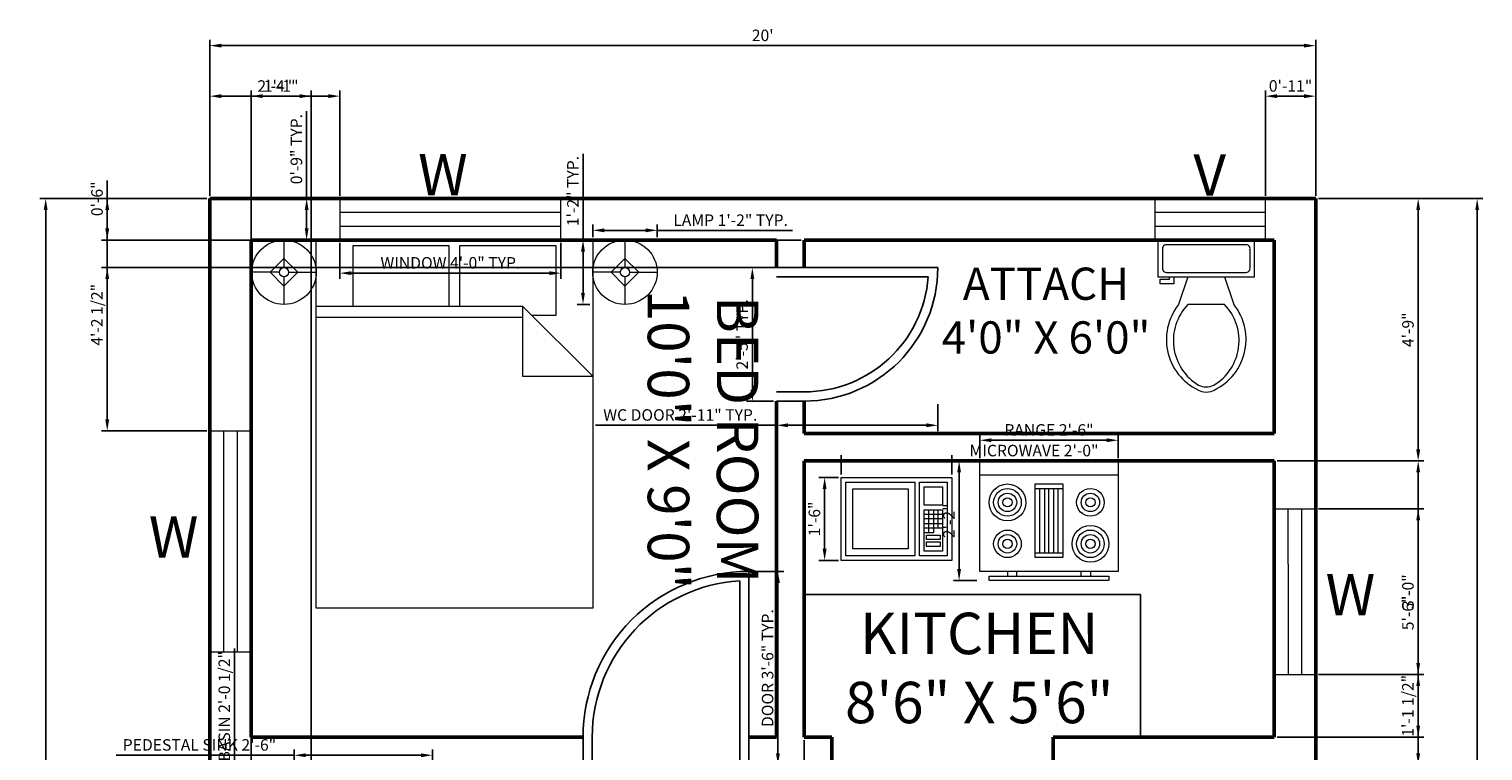
# Model space of a CAD drawing. Units: inches. Extents: x 2530 to 2846, y 1711 to 2145.
# Tile 3 of 3: x 2530 to 2846, y 1989 to 2145. Entities that reach past the tile are written whole.
import ezdxf

# ---------------------------------------------------------------- set-up
doc = ezdxf.new("R2010")
doc.units = ezdxf.units.IN
for name, color, linetype, lineweight in [('A-ANNO-DIMS', 2, 'Continuous', 18), ('A-ANNO-TEXT', 7, 'Continuous', 18), ('A-AREA-IDEN', 7, 'Continuous', 25), ('A-DOOR', 3, 'Continuous', 25), ('A-EQPM', 8, 'Continuous', 18), ('A-FLOR-CASE', 8, 'Continuous', 25), ('A-FLOR-FIXT', 9, 'Continuous', 18), ('A-FURN', 8, 'Continuous', 18), ('A-GLAZ', 4, 'Continuous', 18), ('A-WALL', 7, 'Continuous', 50)]:
    doc.layers.add(name, color=color, linetype=linetype, lineweight=lineweight)
doc.styles.get("Standard").update_dxf_attribs({"font": 'arial.ttf'})
doc.dimstyles.new('ISO-25', dxfattribs={"dimtxt": 2.5, "dimasz": 2.5, "dimexe": 1.25, "dimexo": 0.625, "dimtad": 1, "dimdec": 0, "dimlunit": 3, "dimtxsty": 'Standard', "dimcen": 2.5, "dimadec": 0, "dimazin": 0, "dimtfac": 1, "dimtdec": 0, "dimtmove": 0, "dimatfit": 3, "dimfxl": 1, "dimarcsym": 0})

# ---------------------------------------------------------------- blocks, each defined once
blk = doc.blocks.new('Toilet - top')
for p, q in [((9.5, -6), (9.5, -2)), ((-10, -8.5), (-8, -8.5)), ((-10, -9.5), (-10, -8.5)), ((-8, -8.5), (-8, -8)), ((-7, -8), (-7, -9.5)), ((-4, -8), (-6, -14)), ((4, -8), (6, -14)), ((-7, -9.5), (-10, -9.5)), ((4, -14), (-4, -14))]:
    blk.add_line(p, q)
blk.add_lwpolyline([(10.5, -8), (10.5, 0), (-10.5, 0), (-10.5, -8)], close=True)
for points in [[(-9.5, -2), (-9.5, -6)], [(8.5, -1), (-8.5, -1)], [(-8.5, -7), (8.5, -7)]]:
    blk.add_lwpolyline(points)
for centre, radius, start, end in [((-8.62, -1.88), 0.884, 81.8699, 188.1301), ((8.62, -1.88), 0.884, 351.8699, 98.1301), ((-8.62, -6.12), 0.884, 171.8699, 278.1301), ((8.62, -6.12), 0.884, 261.8699, 8.1301), ((3.52, -21.58), 12.17, 141.4691, 247.9714), ((4.2, -21.82), 11.33, 136.3677, 238.9468), ((-3.52, -21.58), 12.17, 292.0284, 38.5307), ((-4.2, -21.82), 11.33, 301.053, 43.6321), ((0, -27.88), 4, 245.7318, 294.2682), ((0, -29), 4, 254.8605, 285.1395)]:
    blk.add_arc(centre, radius, start, end)
blk = doc.blocks.new('Bed - Queen')
for p, q in [((0, -80.00003), (0, 0)), ((0, 0), (59.99999, 0)), ((59.99999, 0), (59.99999, -80.00003)), ((7.99999, -1.2), (28.79998, -1.2)), ((7.99999, -14.4), (7.99999, -1.2)), ((28.79998, -1.2), (28.79998, -14.4)), ((31.19999, -1.2), (51.99999, -1.2)), ((31.19999, -14.4), (31.19999, -1.2)), ((51.99999, -1.2), (51.99999, -16.4)), ((0, -14.4), (44.8, -14.4)), ((59.99999, -29.6), (44.8, -14.4)), ((44.8, -14.4), (44.8, -29.6)), ((44.8, -16.8), (0, -16.8)), ((51.99999, -16.4), (46.79936, -16.4)), ((44.8, -29.6), (59.99999, -29.6)), ((59.99999, -80.00003), (0, -80.00003))]:
    blk.add_line(p, q)
blk = doc.blocks.new('Lamp - Table')
for p, q in [((0, 7), (0, 1)), ((-1, 0), (-7, 0)), ((0, 3), (-3, 0)), ((-3, 0), (0, -3)), ((3, 0), (0, 3)), ((0, -3), (3, 0)), ((1, 0), (7, 0)), ((0, -1), (0, -7))]:
    blk.add_line(p, q)
for radius in [7, 1]:
    blk.add_circle((0, 0), radius)
blk = doc.blocks.new('Range-Oven - 30 in top')
for p, q in [((0, -3), (30, -3)), ((12, -6), (18, -6)), ((13, -20), (13, -6)), ((14, -6), (14, -20)), ((15, -20), (15, -6)), ((16, -6), (16, -20)), ((17, -20), (17, -6)), ((18, -20), (12, -20)), ((6, -24), (6, -25)), ((8, -25), (8, -24)), ((22, -25), (22, -24)), ((24, -24), (24, -25))]:
    blk.add_line(p, q)
for points in [[(0, -24), (0, 0), (30, 0), (30, -24)], [(12, -21), (12, -5), (18, -5), (18, -21)], [(2, -26), (2, -25), (28, -25), (28, -26)]]:
    blk.add_lwpolyline(points, close=True)
for centre, radius in [((6, -9), 4), ((6, -9), 3), ((24, -9), 3), ((6, -9), 2), ((6, -9), 1), ((24, -9), 2), ((24, -9), 1), ((6, -18), 3), ((24, -18), 4), ((24, -18), 3), ((6, -18), 2), ((6, -18), 1), ((24, -18), 2), ((24, -18), 1)]:
    blk.add_circle(centre, radius)
blk = doc.blocks.new('Microwave')
for p, q in [((18, 10), (22, 10)), ((19, 7), (19, 11)), ((20, 11), (20, 7)), ((21, 7), (21, 11)), ((22, 9), (18, 9)), ((18, 8), (22, 8)), ((22, 7), (18, 7)), ((19, 6), (19, 7)), ((20, 7), (20, 6)), ((20, 6), (18, 6))]:
    blk.add_line(p, q)
for points in [[(0, 0), (0, 18), (24, 18), (24, 0)], [(1, 1), (1, 17), (16, 17), (16, 1)], [(17, 1), (17, 17), (23, 17), (23, 1)], [(18, 12), (18, 16), (22, 16), (22, 12)], [(2.5, 2.5), (2.5, 15.5), (14.5, 15.5), (14.5, 2.5)], [(18, 2), (18, 11), (22, 11), (22, 2)], [(18.5, 4.5), (18.5, 5.5), (21.5, 5.5), (21.5, 4.5)], [(18.5, 3), (18.5, 4), (21.5, 4), (21.5, 3)]]:
    blk.add_lwpolyline(points, close=True)
blk = doc.blocks.new('*D11')
at = {"layer": 'A-ANNO-DIMS', "color": 0, "lineweight": -2, "transparency": 16777216}
for p, q in [((2569.45, 2109.25), (2569.45, 2143.1)), ((2809.45, 2109.25), (2809.45, 2143.1)), ((2571.95, 2141.85), (2806.95, 2141.85))]:
    blk.add_line(p, q, dxfattribs=at)
at = {"layer": 'A-ANNO-DIMS', "color": 0, "transparency": 16777216}
for points in [[(2571.95, 2142.27), (2571.95, 2141.44), (2569.45, 2141.85)], [(2806.95, 2142.27), (2806.95, 2141.44), (2809.45, 2141.85)]]:
    blk.add_solid(points, dxfattribs=at)
at = {"layer": 'Defpoints', "color": 0, "transparency": 16777216}
for p in [(2809.45, 2141.85), (2569.45, 2108.63), (2809.45, 2108.63)]:
    blk.add_point(p, dxfattribs=at)
at = {"layer": 'A-ANNO-DIMS', "color": 0, "transparency": 16777216, "insert": (2689.45, 2143.76), "char_height": 2.5, "width": 0.3496, "attachment_point": 5}
blk.add_mtext("20'", dxfattribs=at)
blk = doc.blocks.new('*D12')
at = {"layer": 'A-ANNO-DIMS', "color": 0, "lineweight": -2, "transparency": 16777216}
for p, q in [((2810.07, 2108.63), (2845.75, 2108.63)), ((2844.5, 2106.13), (2844.5, 1751.13)), ((2810.07, 1748.63), (2845.75, 1748.63))]:
    blk.add_line(p, q, dxfattribs=at)
at = {"layer": 'A-ANNO-DIMS', "color": 0, "transparency": 16777216}
for points in [[(2844.08, 2106.13), (2844.91, 2106.13), (2844.5, 2108.63)], [(2844.08, 1751.13), (2844.91, 1751.13), (2844.5, 1748.63)]]:
    blk.add_solid(points, dxfattribs=at)
at = {"layer": 'Defpoints', "color": 0, "transparency": 16777216}
for p in [(2809.45, 2108.63), (2809.45, 1748.63), (2844.5, 1748.63)]:
    blk.add_point(p, dxfattribs=at)
at = {"layer": 'A-ANNO-DIMS', "color": 0, "transparency": 16777216, "insert": (2842.6, 1928.63), "char_height": 2.5, "attachment_point": 5, "rotation": 90}
blk.add_mtext("30'", dxfattribs=at)
blk = doc.blocks.new('*D13')
at = {"layer": 'A-ANNO-DIMS', "color": 0, "lineweight": -2, "transparency": 16777216}
for p, q in [((2568.82, 2108.63), (2532.59, 2108.63)), ((2533.84, 2106.13), (2533.84, 1751.13)), ((2568.82, 1748.63), (2532.59, 1748.63))]:
    blk.add_line(p, q, dxfattribs=at)
at = {"layer": 'A-ANNO-DIMS', "color": 0, "transparency": 16777216}
for points in [[(2533.43, 2106.13), (2534.26, 2106.13), (2533.84, 2108.63)], [(2533.43, 1751.13), (2534.26, 1751.13), (2533.84, 1748.63)]]:
    blk.add_solid(points, dxfattribs=at)
at = {"layer": 'Defpoints', "color": 0, "transparency": 16777216}
for p in [(2569.45, 2108.63), (2533.84, 1748.63), (2569.45, 1748.63)]:
    blk.add_point(p, dxfattribs=at)
at = {"layer": 'A-ANNO-DIMS', "color": 0, "transparency": 16777216, "insert": (2531.94, 1928.63), "char_height": 2.5, "attachment_point": 5, "rotation": 90}
blk.add_mtext("30'", dxfattribs=at)
blk = doc.blocks.new('WIN-48IN')
for p, q in [((0, 48), (0, 0)), ((9, 48), (0, 48)), ((3, 48), (3, 0)), ((6, 0), (6, 48)), ((9, 0), (9, 48)), ((0, 0), (9, 0))]:
    blk.add_line(p, q)
blk = doc.blocks.new('VENT-24IN')
for p, q in [((24, 9), (0, 9)), ((0, 9), (0, 0)), ((24, 0), (24, 9)), ((24, 6), (0, 6)), ((0, 3), (24, 3)), ((0, 0), (24, 0))]:
    blk.add_line(p, q)
blk = doc.blocks.new('DOOR-SINGLE-29IN')
for p, q in [((0, 35), (0, 29)), ((2, 35), (2, 29)), ((27, 29), (27, 35)), ((29, 29), (29, 35)), ((27, 29), (27, 2.07)), ((29, 29), (29, 0))]:
    blk.add_line(p, q)
for radius, end in [(29, 270), (27, 265.752)]:
    blk.add_arc((29, 29), radius, 180, end)
blk = doc.blocks.new('DOOR-SINGLE-36IN')
for p, q in [((0, 36), (0, 42)), ((2, 36), (2, 42)), ((34, 42), (34, 36)), ((36, 42), (36, 36)), ((0, 36), (0, 0)), ((2, 36), (2, 2.06))]:
    blk.add_line(p, q)
for radius, start in [(36, 270), (34, 273.3723)]:
    blk.add_arc((0, 36), radius, start, 0)
blk = doc.blocks.new('*D20')
at = {"layer": 'A-ANNO-DIMS', "color": 0, "lineweight": -2, "transparency": 16777216}
for p, q in [((2597.67, 2099), (2597.67, 2091.18)), ((2645.67, 2099), (2645.67, 2091.18)), ((2643.17, 2092.43), (2600.17, 2092.43))]:
    blk.add_line(p, q, dxfattribs=at)
at = {"layer": 'A-ANNO-DIMS', "color": 0, "transparency": 16777216}
for points in [[(2600.17, 2092.85), (2600.17, 2092.01), (2597.67, 2092.43)], [(2643.17, 2092.85), (2643.17, 2092.01), (2645.67, 2092.43)]]:
    blk.add_solid(points, dxfattribs=at)
at = {"layer": 'Defpoints', "color": 0, "transparency": 16777216}
for p in [(2597.67, 2099.63), (2645.67, 2099.63), (2597.67, 2092.43)]:
    blk.add_point(p, dxfattribs=at)
at = {"layer": 'A-ANNO-DIMS', "color": 0, "transparency": 16777216, "insert": (2621.67, 2094.35), "char_height": 2.5, "attachment_point": 5}
blk.add_mtext('WINDOW 4\'-0" TYP.', dxfattribs=at)
blk = doc.blocks.new('*D21')
at = {"layer": 'A-ANNO-DIMS', "color": 0, "lineweight": -2, "transparency": 16777216}
for p, q in [((2590.47, 2108.63), (2590.47, 2127.62)), ((2597.05, 2108.63), (2589.22, 2108.63)), ((2590.47, 2102.13), (2590.47, 2106.13)), ((2597.05, 2099.63), (2589.22, 2099.63))]:
    blk.add_line(p, q, dxfattribs=at)
at = {"layer": 'A-ANNO-DIMS', "color": 0, "transparency": 16777216}
for points in [[(2590.06, 2106.13), (2590.89, 2106.13), (2590.47, 2108.63)], [(2590.06, 2102.13), (2590.89, 2102.13), (2590.47, 2099.63)]]:
    blk.add_solid(points, dxfattribs=at)
at = {"layer": 'Defpoints', "color": 0, "transparency": 16777216}
for p in [(2590.47, 2108.63), (2597.67, 2108.63), (2597.67, 2099.63)]:
    blk.add_point(p, dxfattribs=at)
at = {"layer": 'A-ANNO-DIMS', "color": 0, "transparency": 16777216, "insert": (2588.57, 2119.37), "char_height": 2.5, "attachment_point": 5, "rotation": 90}
blk.add_mtext('0\'-9" TYP.', dxfattribs=at)
blk = doc.blocks.new('*D22')
at = {"layer": 'A-ANNO-DIMS', "color": 0, "lineweight": -2, "transparency": 16777216}
for p, q in [((2652.55, 2100.25), (2652.55, 2102.98)), ((2655.05, 2101.73), (2664.05, 2101.73)), ((2666.55, 2100.25), (2666.55, 2102.98)), ((2666.55, 2101.73), (2695.91, 2101.73))]:
    blk.add_line(p, q, dxfattribs=at)
at = {"layer": 'A-ANNO-DIMS', "color": 0, "transparency": 16777216}
for points in [[(2655.05, 2102.15), (2655.05, 2101.31), (2652.55, 2101.73)], [(2664.05, 2102.15), (2664.05, 2101.31), (2666.55, 2101.73)]]:
    blk.add_solid(points, dxfattribs=at)
at = {"layer": 'Defpoints', "color": 0, "transparency": 16777216}
for p in [(2666.55, 2101.73), (2652.55, 2099.63), (2666.55, 2099.63)]:
    blk.add_point(p, dxfattribs=at)
at = {"layer": 'A-ANNO-DIMS', "color": 0, "transparency": 16777216, "insert": (2682.48, 2103.61), "char_height": 2.5, "attachment_point": 5}
blk.add_mtext('LAMP 1\'-2" TYP.', dxfattribs=at)
blk = doc.blocks.new('*D23')
at = {"layer": 'A-ANNO-DIMS', "color": 0, "lineweight": -2, "transparency": 16777216}
for p, q in [((2650.45, 2099.63), (2650.45, 2118.38)), ((2651.92, 2099.63), (2649.2, 2099.63)), ((2650.45, 2088.13), (2650.45, 2097.13)), ((2651.92, 2085.63), (2649.2, 2085.63))]:
    blk.add_line(p, q, dxfattribs=at)
at = {"layer": 'A-ANNO-DIMS', "color": 0, "transparency": 16777216}
for points in [[(2650.03, 2097.13), (2650.86, 2097.13), (2650.45, 2099.63)], [(2650.03, 2088.13), (2650.86, 2088.13), (2650.45, 2085.63)]]:
    blk.add_solid(points, dxfattribs=at)
at = {"layer": 'Defpoints', "color": 0, "transparency": 16777216}
for p in [(2650.45, 2099.63), (2652.55, 2099.63), (2652.55, 2085.63)]:
    blk.add_point(p, dxfattribs=at)
at = {"layer": 'A-ANNO-DIMS', "color": 0, "transparency": 16777216, "insert": (2648.57, 2110.26), "char_height": 2.5, "attachment_point": 5, "rotation": 90}
blk.add_mtext('1\'-2" TYP.', dxfattribs=at)
blk = doc.blocks.new('*D30')
at = {"layer": 'A-ANNO-DIMS', "color": 0, "lineweight": -2, "transparency": 16777216}
for p, q in [((2692.45, 2064), (2692.45, 2058.13)), ((2727.45, 2064), (2727.45, 2058.13)), ((2692.45, 2059.38), (2653.18, 2059.38)), ((2724.95, 2059.38), (2694.95, 2059.38))]:
    blk.add_line(p, q, dxfattribs=at)
at = {"layer": 'A-ANNO-DIMS', "color": 0, "transparency": 16777216}
for points in [[(2694.95, 2059.8), (2694.95, 2058.96), (2692.45, 2059.38)], [(2724.95, 2059.8), (2724.95, 2058.96), (2727.45, 2059.38)]]:
    blk.add_solid(points, dxfattribs=at)
at = {"layer": 'Defpoints', "color": 0, "transparency": 16777216}
for p in [(2692.45, 2064.63), (2727.45, 2064.63), (2692.45, 2059.38)]:
    blk.add_point(p, dxfattribs=at)
at = {"layer": 'A-ANNO-DIMS', "color": 0, "transparency": 16777216, "insert": (2671.56, 2061.3), "char_height": 2.5, "attachment_point": 5}
blk.add_mtext('WC DOOR 2\'-11" TYP.', dxfattribs=at)
blk = doc.blocks.new('*D31')
at = {"layer": 'A-ANNO-DIMS', "color": 0, "lineweight": -2, "transparency": 16777216}
for p, q in [((2691.82, 2093.63), (2685.95, 2093.63)), ((2687.2, 2067.13), (2687.2, 2091.13)), ((2691.82, 2064.63), (2685.95, 2064.63))]:
    blk.add_line(p, q, dxfattribs=at)
at = {"layer": 'A-ANNO-DIMS', "color": 0, "transparency": 16777216}
for points in [[(2686.78, 2091.13), (2687.62, 2091.13), (2687.2, 2093.63)], [(2686.78, 2067.13), (2687.62, 2067.13), (2687.2, 2064.63)]]:
    blk.add_solid(points, dxfattribs=at)
at = {"layer": 'Defpoints', "color": 0, "transparency": 16777216}
for p in [(2687.2, 2093.63), (2692.45, 2093.63), (2692.45, 2064.63)]:
    blk.add_point(p, dxfattribs=at)
at = {"layer": 'A-ANNO-DIMS', "color": 0, "transparency": 16777216, "insert": (2685.3, 2079.13), "char_height": 2.5, "attachment_point": 5, "rotation": 90}
blk.add_mtext('2\'-5" TYP.', dxfattribs=at)
blk = doc.blocks.new('*D32')
at = {"layer": 'A-ANNO-DIMS', "color": 0, "lineweight": -2, "transparency": 16777216}
for p, q in [((2687.07, 2027.63), (2694, 2027.63)), ((2692.75, 2025.13), (2692.75, 1988.13)), ((2687.07, 1985.63), (2694, 1985.63))]:
    blk.add_line(p, q, dxfattribs=at)
at = {"layer": 'A-ANNO-DIMS', "color": 0, "transparency": 16777216}
for points in [[(2692.33, 2025.13), (2693.17, 2025.13), (2692.75, 2027.63)], [(2692.33, 1988.13), (2693.17, 1988.13), (2692.75, 1985.63)]]:
    blk.add_solid(points, dxfattribs=at)
at = {"layer": 'Defpoints', "color": 0, "transparency": 16777216}
for p in [(2686.45, 2027.63), (2686.45, 1985.63), (2692.75, 1985.63)]:
    blk.add_point(p, dxfattribs=at)
at = {"layer": 'A-ANNO-DIMS', "color": 0, "transparency": 16777216, "insert": (2690.83, 2006.63), "char_height": 2.5, "attachment_point": 5, "rotation": 90}
blk.add_mtext('DOOR 3\'-6" TYP.', dxfattribs=at)
blk = doc.blocks.new('*D40')
at = {"layer": 'A-ANNO-DIMS', "color": 0, "lineweight": -2, "transparency": 16777216}
for p, q in [((2736.57, 2052.25), (2736.57, 2057.38)), ((2766.57, 2052.25), (2766.57, 2057.38)), ((2739.07, 2056.13), (2764.07, 2056.13))]:
    blk.add_line(p, q, dxfattribs=at)
at = {"layer": 'A-ANNO-DIMS', "color": 0, "transparency": 16777216}
for points in [[(2739.07, 2056.55), (2739.07, 2055.71), (2736.57, 2056.13)], [(2764.07, 2056.55), (2764.07, 2055.71), (2766.57, 2056.13)]]:
    blk.add_solid(points, dxfattribs=at)
at = {"layer": 'Defpoints', "color": 0, "transparency": 16777216}
for p in [(2766.57, 2056.13), (2736.57, 2051.63), (2766.57, 2051.63)]:
    blk.add_point(p, dxfattribs=at)
at = {"layer": 'A-ANNO-DIMS', "color": 0, "transparency": 16777216, "insert": (2751.57, 2058.05), "char_height": 2.5, "attachment_point": 5}
blk.add_mtext('RANGE 2\'-6"', dxfattribs=at)
blk = doc.blocks.new('*D41')
at = {"layer": 'A-ANNO-DIMS', "color": 0, "lineweight": -2, "transparency": 16777216}
for p, q in [((2735.95, 2051.63), (2730.82, 2051.63)), ((2732.07, 2028.13), (2732.07, 2049.13)), ((2735.95, 2025.63), (2730.82, 2025.63))]:
    blk.add_line(p, q, dxfattribs=at)
at = {"layer": 'A-ANNO-DIMS', "color": 0, "transparency": 16777216}
for points in [[(2731.65, 2049.13), (2732.49, 2049.13), (2732.07, 2051.63)], [(2731.65, 2028.13), (2732.49, 2028.13), (2732.07, 2025.63)]]:
    blk.add_solid(points, dxfattribs=at)
at = {"layer": 'Defpoints', "color": 0, "transparency": 16777216}
for p in [(2732.07, 2051.63), (2736.57, 2051.63), (2736.57, 2025.63)]:
    blk.add_point(p, dxfattribs=at)
at = {"layer": 'A-ANNO-DIMS', "color": 0, "transparency": 16777216, "insert": (2730.19, 2038.63), "char_height": 2.5, "attachment_point": 5, "rotation": 90}
blk.add_mtext('2\'-2"', dxfattribs=at)
blk = doc.blocks.new('*D42')
at = {"layer": 'A-ANNO-DIMS', "color": 0, "lineweight": -2, "transparency": 16777216}
for p, q in [((2706.49, 2048.66), (2706.49, 2052.89)), ((2708.99, 2051.64), (2727.99, 2051.64)), ((2730.49, 2048.66), (2730.49, 2052.89)), ((2730.49, 2051.64), (2763.67, 2051.64))]:
    blk.add_line(p, q, dxfattribs=at)
at = {"layer": 'A-ANNO-DIMS', "color": 0, "transparency": 16777216}
for points in [[(2708.99, 2052.06), (2708.99, 2051.22), (2706.49, 2051.64)], [(2727.99, 2052.06), (2727.99, 2051.22), (2730.49, 2051.64)]]:
    blk.add_solid(points, dxfattribs=at)
at = {"layer": 'Defpoints', "color": 0, "transparency": 16777216}
for p in [(2730.49, 2051.64), (2706.49, 2048.04), (2730.49, 2048.04)]:
    blk.add_point(p, dxfattribs=at)
at = {"layer": 'A-ANNO-DIMS', "color": 0, "transparency": 16777216, "insert": (2748.33, 2053.56), "char_height": 2.5, "attachment_point": 5}
blk.add_mtext('MICROWAVE 2\'-0"', dxfattribs=at)
blk = doc.blocks.new('*D43')
at = {"layer": 'A-ANNO-DIMS', "color": 0, "lineweight": -2, "transparency": 16777216}
for p, q in [((2705.87, 2048.04), (2701.64, 2048.04)), ((2702.89, 2032.54), (2702.89, 2045.54)), ((2705.87, 2030.04), (2701.64, 2030.04))]:
    blk.add_line(p, q, dxfattribs=at)
at = {"layer": 'A-ANNO-DIMS', "color": 0, "transparency": 16777216}
for points in [[(2702.47, 2045.54), (2703.31, 2045.54), (2702.89, 2048.04)], [(2702.47, 2032.54), (2703.31, 2032.54), (2702.89, 2030.04)]]:
    blk.add_solid(points, dxfattribs=at)
at = {"layer": 'Defpoints', "color": 0, "transparency": 16777216}
for p in [(2702.89, 2048.04), (2706.49, 2048.04), (2706.49, 2030.04)]:
    blk.add_point(p, dxfattribs=at)
at = {"layer": 'A-ANNO-DIMS', "color": 0, "transparency": 16777216, "insert": (2700.99, 2039.04), "char_height": 2.5, "attachment_point": 5, "rotation": 90}
blk.add_mtext('1\'-6"', dxfattribs=at)
blk = doc.blocks.new('*D44')
at = {"layer": 'A-ANNO-DIMS', "color": 0, "lineweight": -2, "transparency": 16777216}
for p, q in [((2574.85, 1983.31), (2574.85, 2010.87)), ((2577.91, 1983.31), (2573.6, 1983.31)), ((2574.85, 1961.26), (2574.85, 1980.81)), ((2577.91, 1958.76), (2573.6, 1958.76))]:
    blk.add_line(p, q, dxfattribs=at)
at = {"layer": 'A-ANNO-DIMS', "color": 0, "transparency": 16777216}
for points in [[(2574.43, 1980.81), (2575.27, 1980.81), (2574.85, 1983.31)], [(2574.43, 1961.26), (2575.27, 1961.26), (2574.85, 1958.76)]]:
    blk.add_solid(points, dxfattribs=at)
at = {"layer": 'Defpoints', "color": 0, "transparency": 16777216}
for p in [(2574.85, 1983.31), (2578.53, 1983.31), (2578.53, 1958.76)]:
    blk.add_point(p, dxfattribs=at)
at = {"layer": 'A-ANNO-DIMS', "color": 0, "transparency": 16777216, "insert": (2572.93, 1998.34), "char_height": 2.5, "attachment_point": 5, "rotation": 90}
blk.add_mtext('BASIN 2\'-0 1/2"', dxfattribs=at)
blk = doc.blocks.new('*D46')
at = {"layer": 'A-ANNO-DIMS', "color": 0, "lineweight": -2, "transparency": 16777216}
for p, q in [((2587.77, 1983.82), (2587.77, 1988.95)), ((2617.77, 1983.82), (2617.77, 1988.95)), ((2587.77, 1987.7), (2549.16, 1987.7)), ((2615.27, 1987.7), (2590.27, 1987.7))]:
    blk.add_line(p, q, dxfattribs=at)
at = {"layer": 'A-ANNO-DIMS', "color": 0, "transparency": 16777216}
for points in [[(2590.27, 1988.11), (2590.27, 1987.28), (2587.77, 1987.7)], [(2615.27, 1988.11), (2615.27, 1987.28), (2617.77, 1987.7)]]:
    blk.add_solid(points, dxfattribs=at)
at = {"layer": 'Defpoints', "color": 0, "transparency": 16777216}
for p in [(2587.77, 1987.7), (2587.77, 1983.2), (2617.77, 1983.2)]:
    blk.add_point(p, dxfattribs=at)
at = {"layer": 'A-ANNO-DIMS', "color": 0, "transparency": 16777216, "insert": (2567.21, 1989.62), "char_height": 2.5, "attachment_point": 5}
blk.add_mtext('PEDESTAL SINK 2\'-6"', dxfattribs=at)
blk = doc.blocks.new('*D55')
at = {"layer": 'A-ANNO-DIMS', "color": 0, "lineweight": -2, "transparency": 16777216}
for p, q in [((2801.07, 2051.63), (2832.95, 2051.63)), ((2831.7, 1988.13), (2831.7, 2049.13)), ((2801.07, 1985.63), (2832.95, 1985.63))]:
    blk.add_line(p, q, dxfattribs=at)
at = {"layer": 'A-ANNO-DIMS', "color": 0, "transparency": 16777216}
for points in [[(2831.28, 2049.13), (2832.12, 2049.13), (2831.7, 2051.63)], [(2831.28, 1988.13), (2832.12, 1988.13), (2831.7, 1985.63)]]:
    blk.add_solid(points, dxfattribs=at)
at = {"layer": 'Defpoints', "color": 0, "transparency": 16777216}
for p in [(2800.45, 2051.63), (2831.7, 2051.63), (2800.45, 1985.63)]:
    blk.add_point(p, dxfattribs=at)
at = {"layer": 'A-ANNO-DIMS', "color": 0, "transparency": 16777216, "insert": (2829.8, 2018.63), "char_height": 2.5, "attachment_point": 5, "rotation": 90}
blk.add_mtext('5\'-6"', dxfattribs=at)
blk = doc.blocks.new('*D56')
at = {"layer": 'A-ANNO-DIMS', "color": 0, "lineweight": -2, "transparency": 16777216}
for p, q in [((2810.07, 2108.63), (2832.95, 2108.63)), ((2831.7, 2054.13), (2831.7, 2106.13)), ((2801.07, 2051.63), (2832.95, 2051.63))]:
    blk.add_line(p, q, dxfattribs=at)
at = {"layer": 'A-ANNO-DIMS', "color": 0, "transparency": 16777216}
for points in [[(2831.28, 2106.13), (2832.12, 2106.13), (2831.7, 2108.63)], [(2831.28, 2054.13), (2832.12, 2054.13), (2831.7, 2051.63)]]:
    blk.add_solid(points, dxfattribs=at)
at = {"layer": 'Defpoints', "color": 0, "transparency": 16777216}
for p in [(2809.45, 2108.63), (2831.7, 2108.63), (2800.45, 2051.63)]:
    blk.add_point(p, dxfattribs=at)
at = {"layer": 'A-ANNO-DIMS', "color": 0, "transparency": 16777216, "insert": (2829.8, 2080.13), "char_height": 2.5, "attachment_point": 5, "rotation": 90}
blk.add_mtext('4\'-9"', dxfattribs=at)
blk = doc.blocks.new('*D59')
at = {"layer": 'A-ANNO-DIMS', "color": 0, "lineweight": -2, "transparency": 16777216}
for p, q in [((2810.07, 2041.24), (2832.95, 2041.24)), ((2831.7, 2007.74), (2831.7, 2038.74)), ((2810.07, 2005.24), (2832.95, 2005.24))]:
    blk.add_line(p, q, dxfattribs=at)
at = {"layer": 'A-ANNO-DIMS', "color": 0, "transparency": 16777216}
for points in [[(2831.28, 2038.74), (2832.12, 2038.74), (2831.7, 2041.24)], [(2831.28, 2007.74), (2832.12, 2007.74), (2831.7, 2005.24)]]:
    blk.add_solid(points, dxfattribs=at)
at = {"layer": 'Defpoints', "color": 0, "transparency": 16777216}
for p in [(2809.45, 2041.24), (2831.7, 2041.24), (2809.45, 2005.24)]:
    blk.add_point(p, dxfattribs=at)
at = {"layer": 'A-ANNO-DIMS', "color": 0, "transparency": 16777216, "insert": (2829.8, 2023.24), "char_height": 2.5, "attachment_point": 5, "rotation": 90}
blk.add_mtext('3\'-0"', dxfattribs=at)
blk = doc.blocks.new('*D60')
at = {"layer": 'A-ANNO-DIMS', "color": 0, "lineweight": -2, "transparency": 16777216}
for p, q in [((2810.07, 2005.24), (2832.95, 2005.24)), ((2831.7, 1994.13), (2831.7, 2002.74)), ((2801.07, 1991.63), (2832.95, 1991.63))]:
    blk.add_line(p, q, dxfattribs=at)
at = {"layer": 'A-ANNO-DIMS', "color": 0, "transparency": 16777216}
for points in [[(2831.28, 2002.74), (2832.12, 2002.74), (2831.7, 2005.24)], [(2831.28, 1994.13), (2832.12, 1994.13), (2831.7, 1991.63)]]:
    blk.add_solid(points, dxfattribs=at)
at = {"layer": 'Defpoints', "color": 0, "transparency": 16777216}
for p in [(2809.45, 2005.24), (2831.7, 2005.24), (2800.45, 1991.63)]:
    blk.add_point(p, dxfattribs=at)
at = {"layer": 'A-ANNO-DIMS', "color": 0, "transparency": 16777216, "insert": (2829.78, 1998.44), "char_height": 2.5, "attachment_point": 5, "rotation": 90}
blk.add_mtext('1\'-1 1/2"', dxfattribs=at)
blk = doc.blocks.new('*D62')
at = {"layer": 'A-ANNO-DIMS', "color": 0, "lineweight": -2, "transparency": 16777216}
for p, q in [((2569.45, 2109.25), (2569.45, 2132.13)), ((2571.95, 2130.88), (2595.17, 2130.88)), ((2597.67, 2109.25), (2597.67, 2132.13))]:
    blk.add_line(p, q, dxfattribs=at)
at = {"layer": 'A-ANNO-DIMS', "color": 0, "transparency": 16777216}
for points in [[(2571.95, 2131.3), (2571.95, 2130.46), (2569.45, 2130.88)], [(2595.17, 2131.3), (2595.17, 2130.46), (2597.67, 2130.88)]]:
    blk.add_solid(points, dxfattribs=at)
at = {"layer": 'Defpoints', "color": 0, "transparency": 16777216}
for p in [(2597.67, 2130.88), (2569.45, 2108.63), (2597.67, 2108.63)]:
    blk.add_point(p, dxfattribs=at)
at = {"layer": 'A-ANNO-DIMS', "color": 0, "transparency": 16777216, "insert": (2583.56, 2132.76), "char_height": 2.5, "attachment_point": 5}
blk.add_mtext('2\'-4"', dxfattribs=at)
blk = doc.blocks.new('*D64')
at = {"layer": 'A-ANNO-DIMS', "color": 0, "lineweight": -2, "transparency": 16777216}
for p, q in [((2568.82, 2108.63), (2545.95, 2108.63)), ((2547.2, 2060.64), (2547.2, 2106.13)), ((2568.82, 2058.14), (2545.95, 2058.14))]:
    blk.add_line(p, q, dxfattribs=at)
at = {"layer": 'A-ANNO-DIMS', "color": 0, "transparency": 16777216}
for points in [[(2546.78, 2106.13), (2547.62, 2106.13), (2547.2, 2108.63)], [(2546.78, 2060.64), (2547.62, 2060.64), (2547.2, 2058.14)]]:
    blk.add_solid(points, dxfattribs=at)
at = {"layer": 'Defpoints', "color": 0, "transparency": 16777216}
for p in [(2547.2, 2108.63), (2569.45, 2108.63), (2569.45, 2058.14)]:
    blk.add_point(p, dxfattribs=at)
at = {"layer": 'A-ANNO-DIMS', "color": 0, "transparency": 16777216, "insert": (2545.28, 2083.38), "char_height": 2.5, "attachment_point": 5, "rotation": 90}
blk.add_mtext('4\'-2 1/2"', dxfattribs=at)
blk = doc.blocks.new('*D68')
at = {"layer": 'A-ANNO-DIMS', "color": 0, "lineweight": -2, "transparency": 16777216}
for p, q in [((2578.45, 1950.25), (2578.45, 2132.13)), ((2580.95, 2130.88), (2588.95, 2130.88)), ((2591.45, 1950.25), (2591.45, 2132.13))]:
    blk.add_line(p, q, dxfattribs=at)
at = {"layer": 'A-ANNO-DIMS', "color": 0, "transparency": 16777216}
for points in [[(2580.95, 2131.3), (2580.95, 2130.46), (2578.45, 2130.88)], [(2588.95, 2131.3), (2588.95, 2130.46), (2591.45, 2130.88)]]:
    blk.add_solid(points, dxfattribs=at)
at = {"layer": 'Defpoints', "color": 0, "transparency": 16777216}
for p in [(2591.45, 2130.88), (2578.45, 1949.63), (2591.45, 1949.63)]:
    blk.add_point(p, dxfattribs=at)
at = {"layer": 'A-ANNO-DIMS', "color": 0, "transparency": 16777216, "insert": (2584.95, 2132.76), "char_height": 2.5, "attachment_point": 5}
blk.add_mtext('1\'-1"', dxfattribs=at)
blk = doc.blocks.new('*D69')
at = {"layer": 'A-ANNO-DIMS', "color": 0, "lineweight": -2, "transparency": 16777216}
for p, q in [((2547.2, 2102.13), (2547.2, 2112.53)), ((2697.82, 2099.63), (2545.95, 2099.63)), ((2547.2, 2093.63), (2547.2, 2099.63)), ((2697.82, 2093.63), (2545.95, 2093.63)), ((2547.2, 2091.13), (2547.2, 2088.63))]:
    blk.add_line(p, q, dxfattribs=at)
at = {"layer": 'A-ANNO-DIMS', "color": 0, "transparency": 16777216}
for points in [[(2546.78, 2102.13), (2547.62, 2102.13), (2547.2, 2099.63)], [(2546.78, 2091.13), (2547.62, 2091.13), (2547.2, 2093.63)]]:
    blk.add_solid(points, dxfattribs=at)
at = {"layer": 'Defpoints', "color": 0, "transparency": 16777216}
for p in [(2547.2, 2099.63), (2698.45, 2099.63), (2698.45, 2093.63)]:
    blk.add_point(p, dxfattribs=at)
at = {"layer": 'A-ANNO-DIMS', "color": 0, "transparency": 16777216, "insert": (2545.3, 2108.58), "char_height": 2.5, "attachment_point": 5, "rotation": 90}
blk.add_mtext('0\'-6"', dxfattribs=at)
blk = doc.blocks.new('*D70')
at = {"layer": 'A-ANNO-DIMS', "color": 0, "lineweight": -2, "transparency": 16777216}
for p, q in [((2798.54, 2109.25), (2798.54, 2132.13)), ((2801.04, 2130.88), (2806.95, 2130.88)), ((2809.45, 2109.25), (2809.45, 2132.13))]:
    blk.add_line(p, q, dxfattribs=at)
at = {"layer": 'A-ANNO-DIMS', "color": 0, "transparency": 16777216}
for points in [[(2801.04, 2131.3), (2801.04, 2130.46), (2798.54, 2130.88)], [(2806.95, 2131.3), (2806.95, 2130.46), (2809.45, 2130.88)]]:
    blk.add_solid(points, dxfattribs=at)
at = {"layer": 'Defpoints', "color": 0, "transparency": 16777216}
for p in [(2809.45, 2130.88), (2798.54, 2108.63), (2809.45, 2108.63)]:
    blk.add_point(p, dxfattribs=at)
at = {"layer": 'A-ANNO-DIMS', "color": 0, "transparency": 16777216, "insert": (2804, 2132.78), "char_height": 2.5, "attachment_point": 5}
blk.add_mtext('0\'-11"', dxfattribs=at)
blk = doc.blocks.new('*D72')
at = {"layer": 'A-ANNO-DIMS', "color": 0, "lineweight": -2, "transparency": 16777216}
for p, q in [((2698.45, 1991), (2698.45, 1725.13)), ((2704.45, 1985), (2704.45, 1725.13)), ((2695.95, 1726.38), (2693.45, 1726.38)), ((2698.45, 1726.38), (2704.45, 1726.38)), ((2706.95, 1726.38), (2717.34, 1726.38))]:
    blk.add_line(p, q, dxfattribs=at)
at = {"layer": 'A-ANNO-DIMS', "color": 0, "transparency": 16777216}
for points in [[(2695.95, 1726.8), (2695.95, 1725.96), (2698.45, 1726.38)], [(2706.95, 1726.8), (2706.95, 1725.96), (2704.45, 1726.38)]]:
    blk.add_solid(points, dxfattribs=at)
at = {"layer": 'Defpoints', "color": 0, "transparency": 16777216}
for p in [(2698.45, 1991.63), (2704.45, 1985.63), (2704.45, 1726.38)]:
    blk.add_point(p, dxfattribs=at)
at = {"layer": 'A-ANNO-DIMS', "color": 0, "transparency": 16777216, "insert": (2713.4, 1728.28), "char_height": 2.5, "attachment_point": 5}
blk.add_mtext('0\'-6"', dxfattribs=at)

msp = doc.modelspace()

# ---------------------------------------------------------------- linework, layer by layer
at = {"layer": 'A-FLOR-CASE'}
for p, q in [((2698.45, 2022.63), (2771.45, 2022.63)), ((2771.45, 2022.63), (2771.45, 1991.63))]:
    msp.add_line(p, q, dxfattribs=at)
at = {"layer": 'A-GLAZ'}
for p, q in [((2800.45, 2029.24), (2800.45, 2041.24)), ((2800.45, 2041.24), (2809.45, 2041.24)), ((2803.45, 2029.24), (2803.45, 2041.24)), ((2806.45, 2029.24), (2806.45, 2041.24)), ((2809.45, 2041.24), (2809.45, 2029.24)), ((2800.45, 2029.24), (2800.45, 2005.24)), ((2803.45, 2029.24), (2803.45, 2005.24)), ((2806.45, 2005.24), (2806.45, 2029.24)), ((2809.45, 2005.24), (2809.45, 2029.24)), ((2800.45, 2005.24), (2809.45, 2005.24))]:
    msp.add_line(p, q, dxfattribs=at)
at = {"layer": 'A-WALL'}
for p, q in [((2569.45, 2108.63), (2809.45, 2108.63)), ((2569.45, 1748.63), (2569.45, 2108.63)), ((2809.45, 2108.63), (2809.45, 1748.63)), ((2578.45, 2099.63), (2692.45, 2099.63)), ((2578.45, 1991.63), (2578.45, 2099.63)), ((2692.45, 2099.63), (2692.45, 2093.63)), ((2698.45, 2099.63), (2698.45, 2093.63)), ((2698.45, 2099.63), (2800.45, 2099.63)), ((2698.45, 2099.63), (2698.45, 2093.63)), ((2800.45, 2099.63), (2800.45, 2057.63)), ((2692.45, 2064.63), (2692.45, 1991.63)), ((2698.45, 2064.63), (2698.45, 2057.63)), ((2698.45, 2057.63), (2800.45, 2057.63)), ((2698.45, 2051.63), (2800.45, 2051.63)), ((2698.45, 2051.63), (2698.45, 1991.63)), ((2800.45, 2051.63), (2800.45, 1991.63)), ((2578.45, 1991.63), (2650.45, 1991.63)), ((2692.45, 1991.63), (2686.45, 1991.63)), ((2686.45, 1991.63), (2692.45, 1991.63)), ((2698.45, 1991.63), (2704.45, 1991.63)), ((2698.45, 1991.63), (2704.45, 1991.63)), ((2704.45, 1991.63), (2704.45, 1985.63)), ((2752.45, 1985.63), (2752.45, 1991.63)), ((2752.45, 1991.63), (2800.45, 1991.63))]:
    msp.add_line(p, q, dxfattribs=at)

# ---------------------------------------------------------------- block references
at = {"layer": 'A-DOOR'}
for name, p, rotation in [('DOOR-SINGLE-29IN', (2727.45, 2064.63), 90.00000000000183), ('DOOR-SINGLE-36IN', (2686.45, 2027.63), 180)]:
    msp.add_blockref(name, p, dxfattribs=dict(at, rotation=rotation))
at = {"layer": 'A-EQPM'}
for name, p in [('Range-Oven - 30 in top', (2736.57, 2051.63)), ('Microwave', (2706.49, 2030.04))]:
    msp.add_blockref(name, p, dxfattribs=at)
at = {"layer": 'A-FLOR-FIXT'}
msp.add_blockref('Toilet - top', (2785.7, 2099.6), dxfattribs=at)
at = {"layer": 'A-FURN'}
for name, p in [('Lamp - Table', (2585.55, 2092.63)), ('Bed - Queen', (2592.55, 2099.63)), ('Lamp - Table', (2659.55, 2092.63))]:
    msp.add_blockref(name, p, dxfattribs=at)
at = {"layer": 'A-GLAZ', "rotation": 90.00000000000045}
msp.add_blockref('WIN-48IN', (2645.67, 2099.63), dxfattribs=at)
at = {"layer": 'A-GLAZ'}
for name, p in [('VENT-24IN', (2774.54, 2099.63)), ('WIN-48IN', (2569.45, 2010.13))]:
    msp.add_blockref(name, p, dxfattribs=at)

# ---------------------------------------------------------------- texts
at = {"layer": 'A-ANNO-TEXT', "char_height": 9, "attachment_point": 1}
for s, insert in [('\\pxqc;W', (2588.88, 2118.33)), ('\\pxqc;V', (2755.29, 2118.23)), ('\\pxqc;W', (2530.45, 2039.62)), ('\\pxqc;W', (2785.83, 2027.07))]:
    msp.add_mtext_dynamic_manual_height_columns(s, width=62.3253, gutter_width=12.5, heights=[0], dxfattribs=dict(at, insert=insert))
at = {"layer": 'A-AREA-IDEN', "attachment_point": 1}
for s, width, insert, char_height in [('\\pxqc;ATTACH\\P4\'0" X 6\'0"', 46.9697, (2727.45, 2093.63), 7), ('\\pxqc;KITCHEN ^J8\'6" X 5\'6"', 87.9878, (2692.45, 2018.66), 9)]:
    msp.add_mtext_dynamic_manual_height_columns(s, width=width, gutter_width=12.5, heights=[0], dxfattribs=dict(at, insert=insert, char_height=char_height))
at = {"layer": 'A-AREA-IDEN', "insert": (2688.5, 2100.26), "char_height": 9, "attachment_point": 1, "rotation": 270}
msp.add_mtext_dynamic_manual_height_columns('\\pxqc;BED ROOM\\P10\'0" X 9\'0"', width=87.9878, gutter_width=12.5, heights=[0], dxfattribs=at)

# ---------------------------------------------------------------- dimensions: what is measured, and where the dimension line sits
at = {"layer": 'A-ANNO-DIMS'}
for base, p1, p2, override, picture, middle in [((2809.45, 2141.85), (2569.45, 2108.63), (2809.45, 2108.63), {"dimclrd": 0, "dimclre": 0, "dimclrt": 0}, '*D11', (2689.45, 2143.76)), ((2597.67, 2130.88), (2569.45, 2108.63), (2597.67, 2108.63), {"dimdec": 1, "dimlfac": 1, "dimrnd": 0, "dimzin": 1, "dimdsep": 46, "dimlunit": 4, "dimfrac": 2}, '*D62', (2583.56, 2132.76)), ((2591.45, 2130.88), (2578.45, 1949.63), (2591.45, 1949.63), {"dimdec": 1, "dimlfac": 1, "dimrnd": 0, "dimzin": 1, "dimdsep": 46, "dimlunit": 4, "dimfrac": 2}, '*D68', (2584.95, 2132.76)), ((2809.45, 2130.88), (2798.54, 2108.63), (2809.45, 2108.63), {"dimdec": 1, "dimlfac": 1, "dimrnd": 0, "dimzin": 1, "dimdsep": 46, "dimlunit": 4, "dimfrac": 2}, '*D70', (2804, 2132.78)), ((2704.45, 1726.38), (2698.45, 1991.63), (2704.45, 1985.63), {"dimdec": 1, "dimlfac": 1, "dimrnd": 0, "dimzin": 1, "dimdsep": 46, "dimlunit": 4, "dimfrac": 2}, '*D72', (2713.4, 1728.28))]:
    dim = msp.add_linear_dim(base=base, p1=p1, p2=p2, dimstyle='ISO-25', override=override, dxfattribs=at)
    dim.commit()
    dim.dimension.update_dxf_attribs({"geometry": picture, "text_midpoint": middle})
for base, p1, p2, angle, text, picture, middle in [((2590.47, 2108.63), (2597.67, 2099.63), (2597.67, 2108.63), 90, '<> TYP.', '*D21', (2588.57, 2119.37)), ((2650.45, 2099.63), (2652.55, 2085.63), (2652.55, 2099.63), 90, '<> TYP.', '*D23', (2648.57, 2110.26)), ((2597.67, 2092.43), (2645.67, 2099.63), (2597.67, 2099.63), 180, 'WINDOW <> TYP.', '*D20', (2621.67, 2094.35)), ((2687.2, 2093.63), (2692.45, 2064.63), (2692.45, 2093.63), 90, '<> TYP.', '*D31', (2685.3, 2079.13)), ((2692.45, 2059.38), (2727.45, 2064.63), (2692.45, 2064.63), 180, 'WC DOOR <> TYP.', '*D30', (2671.56, 2061.3)), ((2692.75, 1985.63), (2686.45, 2027.63), (2686.45, 1985.63), 270, 'DOOR <> TYP.', '*D32', (2690.83, 2006.63)), ((2574.8501, 1983.3076), (2578.5327, 1958.7567), (2578.5327, 1983.3076), 90, 'BASIN <>', '*D44', (2572.9325, 1998.3382)), ((2587.77, 1987.7), (2617.77, 1983.2), (2587.77, 1983.2), 180, 'PEDESTAL SINK <>', '*D46', (2567.21, 1989.62))]:
    dim = msp.add_linear_dim(base=base, p1=p1, p2=p2, angle=angle, text=text, dimstyle='ISO-25', override={"dimdec": 1, "dimlfac": 1, "dimrnd": 0, "dimzin": 1, "dimdsep": 46, "dimlunit": 4, "dimfrac": 2}, dxfattribs=at)
    dim.commit()
    dim.dimension.update_dxf_attribs({"geometry": picture, "text_midpoint": middle})
for base, p1, p2, override, picture, middle in [((2547.2, 2099.63), (2698.45, 2093.63), (2698.45, 2099.63), {"dimdec": 1, "dimlfac": 1, "dimrnd": 0, "dimzin": 1, "dimdsep": 46, "dimlunit": 4, "dimfrac": 2}, '*D69', (2545.3, 2108.58)), ((2533.84, 1748.63), (2569.45, 2108.63), (2569.45, 1748.63), {"dimclrd": 0, "dimclre": 0, "dimclrt": 0}, '*D13', (2531.94, 1928.63)), ((2547.2, 2108.63), (2569.45, 2058.14), (2569.45, 2108.63), {"dimdec": 1, "dimlfac": 1, "dimrnd": 0, "dimzin": 1, "dimdsep": 46, "dimlunit": 4, "dimfrac": 2}, '*D64', (2545.28, 2083.38)), ((2831.7, 2108.63), (2800.45, 2051.63), (2809.45, 2108.63), {"dimdec": 1, "dimlfac": 1, "dimrnd": 0, "dimzin": 1, "dimdsep": 46, "dimlunit": 4, "dimfrac": 2}, '*D56', (2829.8, 2080.13)), ((2844.5, 1748.63), (2809.45, 2108.63), (2809.45, 1748.63), {"dimclrd": 0, "dimclre": 0, "dimclrt": 0}, '*D12', (2842.6, 1928.63)), ((2732.07, 2051.63), (2736.57, 2025.63), (2736.57, 2051.63), {"dimdec": 1, "dimlfac": 1, "dimrnd": 0, "dimzin": 1, "dimdsep": 46, "dimlunit": 4, "dimfrac": 2}, '*D41', (2730.19, 2038.63)), ((2831.7, 2051.63), (2800.45, 1985.63), (2800.45, 2051.63), {"dimdec": 1, "dimlfac": 1, "dimrnd": 0, "dimzin": 1, "dimdsep": 46, "dimlunit": 4, "dimfrac": 2}, '*D55', (2829.8, 2018.63)), ((2702.89, 2048.04), (2706.49, 2030.04), (2706.49, 2048.04), {"dimdec": 1, "dimlfac": 1, "dimrnd": 0, "dimzin": 1, "dimdsep": 46, "dimlunit": 4, "dimfrac": 2}, '*D43', (2700.99, 2039.04)), ((2831.7, 2041.24), (2809.45, 2005.24), (2809.45, 2041.24), {"dimdec": 1, "dimlfac": 1, "dimrnd": 0, "dimzin": 1, "dimdsep": 46, "dimlunit": 4, "dimfrac": 2}, '*D59', (2829.8, 2023.24)), ((2831.7, 2005.24), (2800.45, 1991.63), (2809.45, 2005.24), {"dimdec": 1, "dimlfac": 1, "dimrnd": 0, "dimzin": 1, "dimdsep": 46, "dimlunit": 4, "dimfrac": 2}, '*D60', (2829.78, 1998.44))]:
    dim = msp.add_linear_dim(base=base, p1=p1, p2=p2, angle=90, dimstyle='ISO-25', override=override, dxfattribs=at)
    dim.commit()
    dim.dimension.update_dxf_attribs({"geometry": picture, "text_midpoint": middle})
for base, p1, p2, text, picture, middle in [((2666.55, 2101.73), (2652.55, 2099.63), (2666.55, 2099.63), 'LAMP <> TYP.', '*D22', (2682.48, 2103.61)), ((2766.57, 2056.13), (2736.57, 2051.63), (2766.57, 2051.63), 'RANGE <>', '*D40', (2751.57, 2058.05)), ((2730.49, 2051.64), (2706.49, 2048.04), (2730.49, 2048.04), 'MICROWAVE <>', '*D42', (2748.33, 2053.56))]:
    dim = msp.add_linear_dim(base=base, p1=p1, p2=p2, text=text, dimstyle='ISO-25', override={"dimdec": 1, "dimlfac": 1, "dimrnd": 0, "dimzin": 1, "dimdsep": 46, "dimlunit": 4, "dimfrac": 2}, dxfattribs=at)
    dim.commit()
    dim.dimension.update_dxf_attribs({"geometry": picture, "text_midpoint": middle})

doc.saveas('drawing.dxf')
